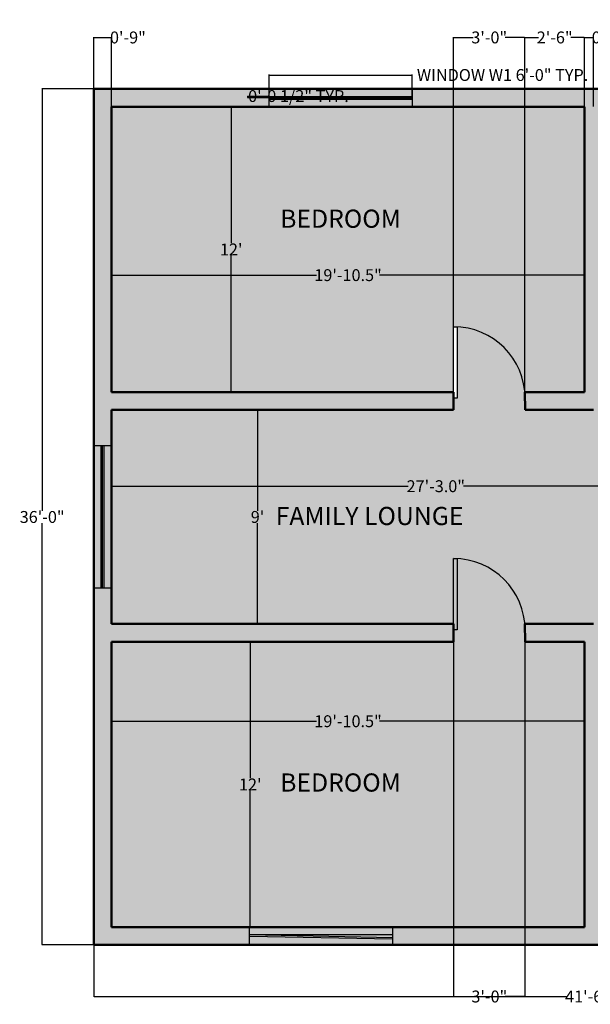
# Model space of a CAD drawing. Units: inches. Extents: x 1379 to 6665, y -118 to 1026.
# Tile 9 of 29: x 2244 to 2532, y 150 to 647. Entities that reach past the tile are written whole.
import ezdxf

# ---------------------------------------------------------------- set-up
doc = ezdxf.new("R2010")
doc.units = ezdxf.units.IN
doc.header["$MEASUREMENT"] = 0
for name, color, linetype, lineweight in [('A-ANNO-DIMS', 2, 'Continuous', 18), ('A-AREA-IDEN', 7, 'Continuous', 25), ('A-DOOR', 1, 'Continuous', 25), ('A-FLOR-PATT', 252, 'Continuous', 13), ('A-GLAZ', 2, 'Continuous', 25), ('A-WALL', 7, 'Continuous', 50), ('A-WALL-PATT', 8, 'Continuous', 13)]:
    doc.layers.add(name, color=color, linetype=linetype, lineweight=lineweight)
doc.styles.get("Standard").update_dxf_attribs({"font": 'arial.ttf'})
doc.dimstyles.get("Standard").update_dxf_attribs({"dimtxt": 6, "dimasz": 0.18, "dimexe": 0.18, "dimexo": 0.0625, "dimgap": 0.09, "dimtad": 0, "dimtih": 1, "dimtoh": 1, "dimdec": 1, "dimzin": 0, "dimdsep": 46, "dimlunit": 3, "dimtxsty": 'Standard', "dimcen": 0.09, "dimclrt": 250, "dimadec": 0, "dimazin": 0, "dimtfac": 1, "dimtdec": 1, "dimtofl": 0, "dimtmove": 0, "dimatfit": 3, "dimfxl": 1, "dimtolj": 1, "dimtzin": 0, "dimarcsym": 0})

# ---------------------------------------------------------------- blocks, each defined once
blk = doc.blocks.new('*U3')
for p, q in [((0, 0), (0, -6)), ((36, 0), (36, -6))]:
    blk.add_line(p, q)
blk.add_lwpolyline([(0, 0), (0, 36), (1.75, 36), (1.75, 0)], close=True)
blk.add_arc((0, 0), 36, 0, 90)
blk = doc.blocks.new('*D26')
at = {"layer": 'A-ANNO-DIMS', "color": 0, "lineweight": -2, "transparency": 16777216}
for p, q in [((2349.32, 602.93), (2350.88, 602.93)), ((2350.7, 602.75), (2350.7, 534.04)), ((2350.7, 459.11), (2350.7, 527.83)), ((2349.32, 458.93), (2350.88, 458.93))]:
    blk.add_line(p, q, dxfattribs=at)
at = {"layer": 'A-ANNO-DIMS', "color": 0, "transparency": 16777216}
for points in [[(2350.67, 602.75), (2350.73, 602.75), (2350.7, 602.93)], [(2350.67, 459.11), (2350.73, 459.11), (2350.7, 458.93)]]:
    blk.add_solid(points, dxfattribs=at)
at = {"layer": 'Defpoints', "color": 0, "transparency": 16777216}
for p in [(2349.26, 602.93), (2349.26, 458.93), (2350.7, 458.93)]:
    blk.add_point(p, dxfattribs=at)
at = {"layer": 'A-ANNO-DIMS', "color": 0, "transparency": 16777216, "insert": (2350.7, 530.93), "char_height": 6, "attachment_point": 5}
blk.add_mtext("\\A1;12'", dxfattribs=at)
blk = doc.blocks.new('*D27')
at = {"layer": 'A-ANNO-DIMS', "color": 0, "lineweight": -2, "transparency": 16777216}
for p, q in [((2290.35, 525.65), (2290.35, 517.8)), ((2528.85, 525.65), (2528.85, 517.8)), ((2290.53, 517.98), (2393.66, 517.98)), ((2528.67, 517.98), (2425.54, 517.98))]:
    blk.add_line(p, q, dxfattribs=at)
at = {"layer": 'A-ANNO-DIMS', "color": 0, "transparency": 16777216}
for points in [[(2290.53, 518.01), (2290.53, 517.95), (2290.35, 517.98)], [(2528.67, 518.01), (2528.67, 517.95), (2528.85, 517.98)]]:
    blk.add_solid(points, dxfattribs=at)
at = {"layer": 'Defpoints', "color": 0, "transparency": 16777216}
for p in [(2290.35, 525.72), (2528.85, 525.72), (2528.85, 517.98)]:
    blk.add_point(p, dxfattribs=at)
at = {"layer": 'A-ANNO-DIMS', "color": 0, "transparency": 16777216, "insert": (2409.6, 517.98), "char_height": 6, "attachment_point": 5}
blk.add_mtext('\\A1;19\'-10.5"', dxfattribs=at)
blk = doc.blocks.new('*D28')
at = {"layer": 'A-ANNO-DIMS', "color": 0, "lineweight": -2, "transparency": 16777216}
for p, q in [((2395.82, 449.93), (2363.77, 449.93)), ((2363.95, 449.75), (2363.95, 399.09)), ((2363.95, 342.11), (2363.95, 392.78)), ((2395.82, 341.93), (2363.77, 341.93))]:
    blk.add_line(p, q, dxfattribs=at)
at = {"layer": 'A-ANNO-DIMS', "color": 0, "transparency": 16777216}
for points in [[(2363.92, 449.75), (2363.98, 449.75), (2363.95, 449.93)], [(2363.92, 342.11), (2363.98, 342.11), (2363.95, 341.93)]]:
    blk.add_solid(points, dxfattribs=at)
at = {"layer": 'Defpoints', "color": 0, "transparency": 16777216}
for p in [(2395.88, 449.93), (2363.95, 341.93), (2395.88, 341.93)]:
    blk.add_point(p, dxfattribs=at)
at = {"layer": 'A-ANNO-DIMS', "color": 0, "transparency": 16777216, "insert": (2363.95, 395.93), "char_height": 6, "attachment_point": 5}
blk.add_mtext("\\A1;9'", dxfattribs=at)
blk = doc.blocks.new('*D29')
at = {"layer": 'A-ANNO-DIMS', "color": 0, "lineweight": -2, "transparency": 16777216}
for p, q in [((2290.35, 390.52), (2290.35, 411.63)), ((2290.53, 411.45), (2439.91, 411.45)), ((2617.17, 411.45), (2467.79, 411.45)), ((2617.35, 390.52), (2617.35, 411.63))]:
    blk.add_line(p, q, dxfattribs=at)
at = {"layer": 'A-ANNO-DIMS', "color": 0, "transparency": 16777216}
for points in [[(2290.53, 411.48), (2290.53, 411.42), (2290.35, 411.45)], [(2617.17, 411.48), (2617.17, 411.42), (2617.35, 411.45)]]:
    blk.add_solid(points, dxfattribs=at)
at = {"layer": 'Defpoints', "color": 0, "transparency": 16777216}
for p in [(2617.35, 411.45), (2290.35, 390.45), (2617.35, 390.45)]:
    blk.add_point(p, dxfattribs=at)
at = {"layer": 'A-ANNO-DIMS', "color": 0, "transparency": 16777216, "insert": (2453.85, 411.45), "char_height": 6, "attachment_point": 5}
blk.add_mtext('\\A1;27\'-3.0"', dxfattribs=at)
blk = doc.blocks.new('*D36')
at = {"layer": 'A-ANNO-DIMS', "color": 0, "lineweight": -2, "transparency": 16777216}
for p, q in [((2376.54, 332.93), (2360.12, 332.93)), ((2360.3, 332.75), (2360.3, 264.04)), ((2360.3, 189.11), (2360.3, 257.83)), ((2376.54, 188.93), (2360.12, 188.93))]:
    blk.add_line(p, q, dxfattribs=at)
at = {"layer": 'A-ANNO-DIMS', "color": 0, "transparency": 16777216}
for points in [[(2360.27, 332.75), (2360.33, 332.75), (2360.3, 332.93)], [(2360.27, 189.11), (2360.33, 189.11), (2360.3, 188.93)]]:
    blk.add_solid(points, dxfattribs=at)
at = {"layer": 'Defpoints', "color": 0, "transparency": 16777216}
for p in [(2376.6, 332.93), (2360.3, 188.93), (2376.6, 188.93)]:
    blk.add_point(p, dxfattribs=at)
at = {"layer": 'A-ANNO-DIMS', "color": 0, "transparency": 16777216, "insert": (2360.3, 260.93), "char_height": 6, "attachment_point": 5}
blk.add_mtext("\\A1;12'", dxfattribs=at)
blk = doc.blocks.new('*D37')
at = {"layer": 'A-ANNO-DIMS', "color": 0, "lineweight": -2, "transparency": 16777216}
for p, q in [((2290.35, 271.73), (2290.35, 293.03)), ((2290.53, 292.85), (2393.66, 292.85)), ((2528.67, 292.85), (2425.54, 292.85)), ((2528.85, 273), (2528.85, 293.03))]:
    blk.add_line(p, q, dxfattribs=at)
at = {"layer": 'A-ANNO-DIMS', "color": 0, "transparency": 16777216}
for points in [[(2290.53, 292.88), (2290.53, 292.82), (2290.35, 292.85)], [(2528.67, 292.88), (2528.67, 292.82), (2528.85, 292.85)]]:
    blk.add_solid(points, dxfattribs=at)
at = {"layer": 'Defpoints', "color": 0, "transparency": 16777216}
for p in [(2528.85, 292.85), (2290.35, 271.66), (2528.85, 272.93)]:
    blk.add_point(p, dxfattribs=at)
at = {"layer": 'A-ANNO-DIMS', "color": 0, "transparency": 16777216, "insert": (2409.6, 292.85), "char_height": 6, "attachment_point": 5}
blk.add_mtext('\\A1;19\'-10.5"', dxfattribs=at)
blk = doc.blocks.new('WIN-1800')
for p, q in [((0, 0.73), (72, 0.73)), ((0, 0), (72, 0))]:
    blk.add_line(p, q)
blk = doc.blocks.new('*D111')
at = {"layer": 'A-ANNO-DIMS', "color": 0, "lineweight": -2, "transparency": 16777216}
for p, q in [((2369.85, 608.23), (2369.85, 619.15)), ((2370.03, 618.97), (2441.67, 618.97)), ((2441.85, 608.23), (2441.85, 619.15)), ((2441.85, 618.97), (2442.03, 618.97))]:
    blk.add_line(p, q, dxfattribs=at)
at = {"layer": 'A-ANNO-DIMS', "color": 0, "transparency": 16777216}
for points in [[(2370.03, 619), (2370.03, 618.94), (2369.85, 618.97)], [(2441.67, 619), (2441.67, 618.94), (2441.85, 618.97)]]:
    blk.add_solid(points, dxfattribs=at)
at = {"layer": 'Defpoints', "color": 0, "transparency": 16777216}
for p in [(2441.85, 618.97), (2369.85, 608.17), (2441.85, 608.17)]:
    blk.add_point(p, dxfattribs=at)
at = {"layer": 'A-ANNO-DIMS', "color": 250, "transparency": 16777216, "insert": (2487.53, 618.97), "char_height": 6, "attachment_point": 5}
blk.add_mtext('\\A1;WINDOW W1 6\'-0" TYP.', dxfattribs=at)
blk = doc.blocks.new('*D112')
at = {"layer": 'A-ANNO-DIMS', "color": 0, "lineweight": -2, "transparency": 16777216}
for p, q in [((2369.79, 608.17), (2358.87, 608.17)), ((2369.79, 607.43), (2358.87, 607.43)), ((2359.05, 608.17), (2359.05, 608.35)), ((2359.05, 608.35), (2359.23, 608.35)), ((2359.05, 607.61), (2359.05, 607.99))]:
    blk.add_line(p, q, dxfattribs=at)
at = {"layer": 'A-ANNO-DIMS', "color": 0, "transparency": 16777216}
for points in [[(2359.02, 607.99), (2359.08, 607.99), (2359.05, 608.17)], [(2359.02, 607.61), (2359.08, 607.61), (2359.05, 607.43)]]:
    blk.add_solid(points, dxfattribs=at)
at = {"layer": 'Defpoints', "color": 0, "transparency": 16777216}
for p in [(2359.05, 608.17), (2369.85, 608.17), (2369.85, 607.43)]:
    blk.add_point(p, dxfattribs=at)
at = {"layer": 'A-ANNO-DIMS', "color": 250, "transparency": 16777216, "insert": (2384.6, 608.35), "char_height": 6, "attachment_point": 5}
blk.add_mtext('\\A1;0\'-0 1/2" TYP.', dxfattribs=at)
blk = doc.blocks.new('*D152')
at = {"layer": 'A-ANNO-DIMS', "color": 0, "lineweight": -2, "transparency": 16777216}
for p, q in [((2281.35, 179.87), (2281.35, 153.75)), ((2779.35, 179.87), (2779.35, 153.75)), ((2281.53, 153.93), (2519.83, 153.93)), ((2779.17, 153.93), (2540.87, 153.93))]:
    blk.add_line(p, q, dxfattribs=at)
at = {"layer": 'A-ANNO-DIMS', "color": 0, "transparency": 16777216}
for points in [[(2281.53, 153.96), (2281.53, 153.9), (2281.35, 153.93)], [(2779.17, 153.96), (2779.17, 153.9), (2779.35, 153.93)]]:
    blk.add_solid(points, dxfattribs=at)
at = {"layer": 'Defpoints', "color": 0, "transparency": 16777216}
for p in [(2281.35, 179.93), (2779.35, 179.93), (2779.35, 153.93)]:
    blk.add_point(p, dxfattribs=at)
at = {"layer": 'A-ANNO-DIMS', "color": 250, "transparency": 16777216, "insert": (2530.35, 153.93), "char_height": 6, "attachment_point": 5}
blk.add_mtext('\\A1;41\'-6"', dxfattribs=at)
blk = doc.blocks.new('*D153')
at = {"layer": 'A-ANNO-DIMS', "color": 0, "lineweight": -2, "transparency": 16777216}
for p, q in [((2281.29, 611.93), (2255.17, 611.93)), ((2255.35, 611.75), (2255.35, 399.09)), ((2255.35, 180.11), (2255.35, 392.78)), ((2281.29, 179.93), (2255.17, 179.93))]:
    blk.add_line(p, q, dxfattribs=at)
at = {"layer": 'A-ANNO-DIMS', "color": 0, "transparency": 16777216}
for points in [[(2255.32, 611.75), (2255.38, 611.75), (2255.35, 611.93)], [(2255.32, 180.11), (2255.38, 180.11), (2255.35, 179.93)]]:
    blk.add_solid(points, dxfattribs=at)
at = {"layer": 'Defpoints', "color": 0, "transparency": 16777216}
for p in [(2255.35, 611.93), (2281.35, 611.93), (2281.35, 179.93)]:
    blk.add_point(p, dxfattribs=at)
at = {"layer": 'A-ANNO-DIMS', "color": 250, "transparency": 16777216, "insert": (2255.35, 395.93), "char_height": 6, "attachment_point": 5}
blk.add_mtext('\\A1;36\'-0"', dxfattribs=at)
blk = doc.blocks.new('*D154')
at = {"layer": 'A-ANNO-DIMS', "color": 0, "lineweight": -2, "transparency": 16777216}
for p, q in [((2281.35, 612), (2281.35, 638.11)), ((2281.53, 637.93), (2290.17, 637.93)), ((2290.35, 603), (2290.35, 638.11)), ((2290.35, 637.93), (2290.53, 637.93))]:
    blk.add_line(p, q, dxfattribs=at)
at = {"layer": 'A-ANNO-DIMS', "color": 0, "transparency": 16777216}
for points in [[(2281.53, 637.96), (2281.53, 637.9), (2281.35, 637.93)], [(2290.17, 637.96), (2290.17, 637.9), (2290.35, 637.93)]]:
    blk.add_solid(points, dxfattribs=at)
at = {"layer": 'Defpoints', "color": 0, "transparency": 16777216}
for p in [(2290.35, 637.93), (2281.35, 611.93), (2290.35, 602.93)]:
    blk.add_point(p, dxfattribs=at)
at = {"layer": 'A-ANNO-DIMS', "color": 250, "transparency": 16777216, "insert": (2298.6, 637.93), "char_height": 6, "attachment_point": 5}
blk.add_mtext('\\A1;0\'-9"', dxfattribs=at)
blk = doc.blocks.new('*D155')
at = {"layer": 'A-ANNO-DIMS', "color": 0, "lineweight": -2, "transparency": 16777216}
for p, q in [((2528.85, 603), (2528.85, 638.11)), ((2529.03, 637.93), (2533.17, 637.93)), ((2533.35, 603), (2533.35, 638.11)), ((2533.35, 637.93), (2533.53, 637.93))]:
    blk.add_line(p, q, dxfattribs=at)
at = {"layer": 'A-ANNO-DIMS', "color": 0, "transparency": 16777216}
for points in [[(2529.03, 637.96), (2529.03, 637.9), (2528.85, 637.93)], [(2533.17, 637.96), (2533.17, 637.9), (2533.35, 637.93)]]:
    blk.add_solid(points, dxfattribs=at)
at = {"layer": 'Defpoints', "color": 0, "transparency": 16777216}
for p in [(2533.35, 637.93), (2528.85, 602.93), (2533.35, 602.93)]:
    blk.add_point(p, dxfattribs=at)
at = {"layer": 'A-ANNO-DIMS', "color": 250, "transparency": 16777216, "insert": (2548.59, 637.93), "char_height": 6, "attachment_point": 5}
blk.add_mtext('\\A1;0\'-4 1/2"', dxfattribs=at)
blk = doc.blocks.new('*D159')
at = {"layer": 'A-ANNO-DIMS', "color": 0, "lineweight": -2, "transparency": 16777216}
for p, q in [((2498.73, 459), (2498.73, 638.11)), ((2498.91, 637.93), (2505.67, 637.93)), ((2528.67, 637.93), (2521.9, 637.93)), ((2528.85, 459), (2528.85, 638.11))]:
    blk.add_line(p, q, dxfattribs=at)
at = {"layer": 'A-ANNO-DIMS', "color": 0, "transparency": 16777216}
for points in [[(2498.91, 637.96), (2498.91, 637.9), (2498.73, 637.93)], [(2528.67, 637.96), (2528.67, 637.9), (2528.85, 637.93)]]:
    blk.add_solid(points, dxfattribs=at)
at = {"layer": 'Defpoints', "color": 0, "transparency": 16777216}
for p in [(2528.85, 637.93), (2498.73, 458.93), (2528.85, 458.93)]:
    blk.add_point(p, dxfattribs=at)
at = {"layer": 'A-ANNO-DIMS', "color": 250, "transparency": 16777216, "insert": (2513.79, 637.93), "char_height": 6, "attachment_point": 5}
blk.add_mtext('\\A1;2\'-6"', dxfattribs=at)
blk = doc.blocks.new('*D160')
at = {"layer": 'A-ANNO-DIMS', "color": 0, "lineweight": -2, "transparency": 16777216}
for p, q in [((2462.85, 459), (2462.85, 638.11)), ((2463.03, 637.93), (2472.73, 637.93)), ((2498.55, 637.93), (2488.85, 637.93)), ((2498.73, 459), (2498.73, 638.11))]:
    blk.add_line(p, q, dxfattribs=at)
at = {"layer": 'A-ANNO-DIMS', "color": 0, "transparency": 16777216}
for points in [[(2463.03, 637.96), (2463.03, 637.9), (2462.85, 637.93)], [(2498.55, 637.96), (2498.55, 637.9), (2498.73, 637.93)]]:
    blk.add_solid(points, dxfattribs=at)
at = {"layer": 'Defpoints', "color": 0, "transparency": 16777216}
for p in [(2498.73, 637.93), (2462.85, 458.93), (2498.73, 458.93)]:
    blk.add_point(p, dxfattribs=at)
at = {"layer": 'A-ANNO-DIMS', "color": 250, "transparency": 16777216, "insert": (2480.79, 637.93), "char_height": 6, "attachment_point": 5}
blk.add_mtext('\\A1;3\'-0"', dxfattribs=at)
blk = doc.blocks.new('*D161')
at = {"layer": 'A-ANNO-DIMS', "color": 0, "lineweight": -2, "transparency": 16777216}
for p, q in [((2462.85, 341.87), (2462.85, 153.75)), ((2498.82, 341.87), (2498.82, 153.75)), ((2463.03, 153.93), (2472.77, 153.93)), ((2498.64, 153.93), (2488.9, 153.93))]:
    blk.add_line(p, q, dxfattribs=at)
at = {"layer": 'A-ANNO-DIMS', "color": 0, "transparency": 16777216}
for points in [[(2463.03, 153.96), (2463.03, 153.9), (2462.85, 153.93)], [(2498.64, 153.96), (2498.64, 153.9), (2498.82, 153.93)]]:
    blk.add_solid(points, dxfattribs=at)
at = {"layer": 'Defpoints', "color": 0, "transparency": 16777216}
for p in [(2462.85, 341.93), (2498.82, 341.93), (2498.82, 153.93)]:
    blk.add_point(p, dxfattribs=at)
at = {"layer": 'A-ANNO-DIMS', "color": 250, "transparency": 16777216, "insert": (2480.83, 153.93), "char_height": 6, "attachment_point": 5}
blk.add_mtext('\\A1;3\'-0"', dxfattribs=at)

msp = doc.modelspace()

# ---------------------------------------------------------------- hatches: boundary and pattern name
at = {"layer": 'A-FLOR-PATT', "transparency": 33554590}
h = msp.add_hatch(color=256, dxfattribs=at)
h.dxf.hatch_style = 1
h.paths.add_polyline_path([(2290.35, 490.43), (2290.35, 602.93), (2369.85, 602.93), (2369.85, 611.93), (2281.35, 611.93), (2281.35, 499.43), (2281.35, 431.93), (2290.35, 431.93), (2290.35, 449.93), (2462.85, 449.93), (2462.85, 458.93), (2290.35, 458.93)])
h.paths.add_polyline_path([(2462.85, 341.93), (2290.35, 341.93), (2290.35, 359.93), (2281.35, 359.93), (2281.35, 179.93), (2359.96, 179.93), (2359.96, 188.93), (2290.35, 188.93), (2290.35, 332.93), (2462.85, 332.93)])
h.paths.add_polyline_path([(2557.35, 188.93), (2533.35, 188.93), (2533.35, 272.93), (2581.35, 272.93), (2581.35, 277.43), (2533.35, 277.43), (2533.35, 332.93), (2533.35, 341.93), (2498.82, 341.93), (2498.85, 332.93), (2528.85, 332.93), (2528.85, 188.93), (2431.96, 188.93), (2431.96, 179.93), (2557.35, 179.93)])
h.paths.add_polyline_path([(2666.85, 188.93), (2614.35, 188.93), (2614.35, 277.43), (2605.35, 277.43), (2605.35, 272.93), (2605.35, 188.93), (2581.35, 188.93), (2581.35, 179.93), (2617.35, 179.93), (2666.85, 179.93)])
h.paths.add_polyline_path([(2779.35, 296.93), (2770.35, 296.93), (2770.35, 284.93), (2740.35, 284.93), (2740.35, 280.43), (2770.35, 280.43), (2770.35, 188.93), (2738.85, 188.93), (2738.85, 179.93), (2779.35, 179.93)])
h.paths.add_polyline_path([(2779.35, 611.93), (2728.35, 611.93), (2728.35, 602.93), (2770.35, 602.93), (2770.35, 482.93), (2722.35, 482.93), (2722.35, 478.43), (2770.35, 478.43), (2770.35, 439.43), (2626.35, 439.43), (2617.35, 439.43), (2617.35, 430.43), (2617.35, 425.93), (2770.35, 425.93), (2770.35, 341.93), (2617.35, 341.93), (2569.35, 341.93), (2569.35, 332.93), (2617.35, 332.93), (2681.85, 332.93), (2681.85, 284.93), (2654.35, 284.93), (2654.35, 280.43), (2681.85, 280.43), (2716.35, 280.43), (2716.35, 284.93), (2686.35, 284.93), (2686.35, 332.93), (2770.35, 332.93), (2770.35, 320.93), (2779.35, 320.93)])
h.paths.add_polyline_path([(2698.35, 482.93), (2650.35, 482.93), (2650.35, 478.43), (2650.35, 439.43), (2654.85, 439.43), (2654.85, 478.43), (2698.35, 478.43)], flags=17)
h.paths.add_polyline_path([(2614.35, 602.93), (2656.35, 602.93), (2656.35, 611.93), (2581.35, 611.93), (2581.35, 602.93), (2605.35, 602.93), (2605.35, 478.43), (2614.35, 478.43), (2614.35, 482.93)], flags=17)
h.paths.add_polyline_path([(2557.35, 611.93), (2521.35, 611.93), (2441.85, 611.93), (2441.85, 602.93), (2521.35, 602.93), (2528.85, 602.93), (2528.85, 458.93), (2498.73, 458.93), (2498.85, 449.93), (2533.35, 449.93), (2533.35, 514.43), (2581.35, 514.43), (2581.35, 518.93), (2533.35, 518.93), (2533.35, 602.93), (2557.35, 602.93)])
at = {"layer": 'A-WALL-PATT', "transparency": 33554564}
h = msp.add_hatch(color=256, dxfattribs=at)
h.dxf.hatch_style = 1
h.paths.add_polyline_path([(2441.85, 611.93), (2369.85, 611.93), (2369.85, 608.17), (2441.85, 608.17)])
h.paths.add_polyline_path([(2441.85, 607.43), (2369.85, 607.43), (2369.85, 606.7), (2441.85, 606.7)])
h.paths.add_polyline_path([(2441.85, 608.17), (2369.85, 608.17), (2369.85, 607.43), (2441.85, 607.43)])
h.paths.add_polyline_path([(2441.85, 606.7), (2369.85, 606.7), (2369.85, 602.93), (2441.85, 602.93)])
at = {"layer": 'A-WALL-PATT', "transparency": 33554590}
h = msp.add_hatch(color=256, dxfattribs=at)
h.dxf.hatch_style = 1
h.paths.add_polyline_path([(2528.85, 602.93), (2290.35, 602.93), (2290.35, 490.43), (2290.35, 458.93), (2462.85, 458.93), (2462.85, 491.93), (2464.6, 491.93), (2464.6, 491.89, -0.376042), (2498.73, 458.93), (2528.85, 458.93)])
h.paths.add_polyline_path([(2617.35, 425.93), (2617.35, 430.43), (2617.35, 439.43), (2626.35, 439.43), (2650.35, 439.43), (2650.35, 478.43), (2650.35, 484.43, 0.400041), (2616.1, 520.39), (2616.1, 484.43), (2614.35, 484.43), (2614.35, 478.43), (2605.35, 478.43), (2605.35, 522.68, 0.392996), (2583.1, 546.62), (2583.1, 522.68), (2581.35, 522.68), (2581.35, 516.68), (2581.35, 514.43), (2533.35, 514.43), (2533.35, 449.93), (2498.85, 449.93), (2498.73, 458.93, 0.376042), (2464.6, 491.89), (2464.6, 455.93), (2462.85, 455.93), (2462.85, 449.93), (2290.35, 449.93), (2290.35, 341.93), (2462.85, 341.93), (2462.85, 374.93), (2464.6, 374.93), (2464.6, 374.89, -0.376042), (2498.73, 341.93), (2533.35, 341.93), (2533.35, 332.93), (2533.35, 277.43), (2581.35, 277.43), (2581.35, 281.18), (2581.35, 305.18), (2583.1, 305.18), (2583.1, 305.12, -0.392996), (2605.35, 281.18), (2605.35, 277.43), (2614.35, 277.43), (2614.35, 283.43), (2614.35, 323.43), (2616.1, 323.43), (2616.1, 323.4, -0.390605), (2654.32, 284.93), (2681.85, 284.93), (2681.85, 332.93), (2614.35, 332.93), (2569.35, 332.93), (2569.35, 341.93), (2617.35, 341.93), (2617.35, 383.93)])
h.paths.add_polyline_path([(2605.35, 602.93), (2533.35, 602.93), (2533.35, 518.93), (2581.35, 518.93), (2581.35, 522.68), (2581.35, 546.68), (2583.1, 546.68), (2583.1, 546.62, -0.392996), (2605.35, 522.68)])
h.paths.add_polyline_path([(2770.35, 602.93), (2614.35, 602.93), (2614.35, 520.43), (2616.1, 520.43), (2616.1, 520.39, -0.400041), (2650.35, 484.43), (2650.35, 482.93), (2698.35, 482.93), (2698.35, 484.43), (2698.35, 508.43), (2700.1, 508.43), (2700.1, 508.37, -0.392996), (2722.35, 484.43), (2722.35, 482.93), (2770.35, 482.93)])
h.paths.add_polyline_path([(2528.85, 332.93), (2498.85, 332.93), (2498.82, 341.93), (2498.73, 341.93, 0.376042), (2464.6, 374.89), (2464.6, 374.93), (2462.85, 374.93), (2462.85, 341.93), (2462.85, 332.93), (2290.35, 332.93), (2290.35, 188.93), (2528.85, 188.93)])
h.paths.add_polyline_path([(2605.35, 272.93), (2605.35, 277.43), (2605.35, 281.18, 0.392996), (2583.1, 305.12), (2583.1, 281.18), (2581.35, 281.18), (2581.35, 277.43), (2581.35, 275.18), (2581.35, 272.93), (2533.35, 272.93), (2533.35, 188.93), (2605.35, 188.93)])
h.paths.add_polyline_path([(2770.35, 280.43), (2740.35, 280.43), (2740.35, 286.43, 0.392996), (2718.1, 310.37), (2718.1, 286.43), (2716.35, 286.43), (2716.35, 280.43), (2681.85, 280.43), (2654.35, 280.43), (2654.35, 283.43, 0.401453), (2616.1, 323.4), (2616.1, 283.43), (2614.35, 283.43), (2614.35, 277.43), (2614.35, 188.93), (2617.35, 188.93), (2770.35, 188.93)])
h.paths.add_polyline_path([(2770.35, 332.93), (2686.35, 332.93), (2686.35, 284.93), (2716.35, 284.93), (2716.35, 286.43), (2716.35, 310.43), (2718.1, 310.43), (2718.1, 310.37, -0.392996), (2740.35, 286.43), (2740.35, 284.93), (2770.35, 284.93)])
h.paths.add_polyline_path([(2770.35, 478.43), (2722.35, 478.43), (2722.35, 484.43, 0.392996), (2700.1, 508.37), (2700.1, 484.43), (2698.35, 484.43), (2698.35, 482.93), (2698.35, 478.43), (2654.85, 478.43), (2654.85, 439.43), (2770.35, 439.43)])
h.paths.add_polyline_path([(2372.98, 539.34), (2443.91, 539.34), (2443.91, 553.57), (2372.98, 553.57)], flags=24)
h.paths.add_polyline_path([(2370.72, 389.31), (2479.4, 389.31), (2479.4, 403.55), (2370.72, 403.55)], flags=24)
h.paths.add_polyline_path([(2550.99, 562.74), (2600.58, 562.74), (2600.58, 576.98), (2550.99, 576.98)], flags=24)
h.paths.add_polyline_path([(2663.19, 559.03), (2734.13, 559.03), (2734.13, 573.27), (2663.19, 573.27)], flags=24)
h.paths.add_polyline_path([(2372.98, 254.81), (2443.91, 254.81), (2443.91, 269.04), (2372.98, 269.04)], flags=24)
h.paths.add_polyline_path([(2545.25, 230.45), (2594.84, 230.45), (2594.84, 244.68), (2545.25, 244.68)], flags=24)
h.paths.add_polyline_path([(2664.48, 230.74), (2735.42, 230.74), (2735.42, 244.97), (2664.48, 244.97)], flags=24)
h.paths.add_polyline_path([(2704.72, 315.06), (2754.31, 315.06), (2754.31, 329.29), (2704.72, 329.29)], flags=24)
h.paths.add_polyline_path([(2688.89, 449.86), (2738.48, 449.86), (2738.48, 464.09), (2688.89, 464.09)], flags=24)
at = {"layer": 'A-WALL-PATT', "transparency": 33554564}
h = msp.add_hatch(color=256, dxfattribs=at)
h.dxf.hatch_style = 1
h.paths.add_polyline_path([(2281.35, 431.93), (2281.35, 359.93), (2285.12, 359.93), (2285.12, 431.93)])
h.paths.add_polyline_path([(2285.85, 431.93), (2285.85, 359.93), (2286.58, 359.93), (2286.58, 431.93)])
h.paths.add_polyline_path([(2285.12, 431.93), (2285.12, 359.93), (2285.85, 359.93), (2285.85, 431.93)])
h.paths.add_polyline_path([(2286.58, 431.93), (2286.58, 359.93), (2290.35, 359.93), (2290.35, 431.93)])
h = msp.add_hatch(color=256, dxfattribs=at)
h.dxf.hatch_style = 1
h.paths.add_polyline_path([(2431.96, 188.93), (2359.96, 188.93), (2359.96, 185.17), (2431.96, 185.17)])
h.paths.add_polyline_path([(2431.96, 184.43), (2359.96, 184.43), (2359.96, 183.7), (2431.96, 183.7)])
h.paths.add_polyline_path([(2431.96, 185.17), (2359.96, 185.17), (2359.96, 184.43), (2431.96, 184.43)])
h.paths.add_polyline_path([(2431.96, 183.7), (2359.96, 183.7), (2359.96, 179.93), (2431.96, 179.93)])

# ---------------------------------------------------------------- linework, layer by layer
at = {"layer": 'A-GLAZ'}
for p, q in [((2369.85, 606.7), (2441.85, 606.7)), ((2285.12, 359.93), (2285.12, 431.93)), ((2285.85, 359.93), (2285.85, 431.93)), ((2286.58, 359.93), (2286.58, 431.93)), ((2359.96, 185.17), (2431.96, 185.17))]:
    msp.add_line(p, q, dxfattribs=at)
for points in [[(2369.85, 611.93), (2441.85, 611.93), (2441.85, 602.93), (2369.85, 602.93)], [(2281.35, 359.93), (2281.35, 431.93), (2290.35, 431.93), (2290.35, 359.93)], [(2359.96, 188.93), (2431.96, 188.93), (2431.96, 179.93), (2359.96, 179.93)]]:
    msp.add_lwpolyline(points, close=True, dxfattribs=at)
at = {"layer": 'A-WALL'}
for p, q in [((2281.35, 499.43), (2281.35, 611.93)), ((2281.35, 611.93), (2521.35, 611.93)), ((2779.35, 611.93), (2521.35, 611.93)), ((2290.35, 602.93), (2521.35, 602.93)), ((2290.35, 490.43), (2290.35, 602.93)), ((2528.85, 602.93), (2290.35, 602.93)), ((2528.85, 458.93), (2528.85, 602.93)), ((2281.35, 499.43), (2281.35, 179.93)), ((2290.35, 490.43), (2290.35, 458.93)), ((2462.85, 458.93), (2290.35, 458.93)), ((2462.85, 449.93), (2462.85, 458.93)), ((2528.85, 458.93), (2498.73, 458.93)), ((2498.85, 449.93), (2498.73, 458.93)), ((2462.85, 449.93), (2290.35, 449.93)), ((2290.35, 449.93), (2290.35, 341.93)), ((2533.35, 449.93), (2498.85, 449.93)), ((2462.85, 341.93), (2290.35, 341.93)), ((2462.85, 332.93), (2462.85, 341.93)), ((2533.35, 341.93), (2498.82, 341.93)), ((2498.82, 341.93), (2498.85, 332.93)), ((2462.85, 332.93), (2290.35, 332.93)), ((2290.35, 332.93), (2290.35, 188.93)), ((2528.85, 332.93), (2498.85, 332.93)), ((2528.85, 332.93), (2528.85, 188.93)), ((2528.85, 188.93), (2290.35, 188.93)), ((2617.35, 179.93), (2281.35, 179.93))]:
    msp.add_line(p, q, dxfattribs=at)

# ---------------------------------------------------------------- block references
at = {"layer": 'A-DOOR'}
for p in [(2462.85, 455.93), (2462.85, 338.93)]:
    msp.add_blockref('*U3', p, dxfattribs=at)
at = {"layer": 'A-GLAZ'}
msp.add_blockref('WIN-1800', (2369.85, 607.43), dxfattribs=at)
at = {"layer": 'A-GLAZ', "rotation": 358.834332312017}
msp.add_blockref('WIN-1800', (2359.96, 184.43), dxfattribs=at)

# ---------------------------------------------------------------- texts
at = {"layer": 'A-AREA-IDEN'}
for s, height, p in [('BEDROOM', 9.17, (2375.35, 541.87)), ('FAMILY LOUNGE', 9.1702, (2373.1, 391.84)), ('BEDROOM', 9.17, (2375.35, 257.34))]:
    msp.add_text(s, height=height, dxfattribs=at).set_placement(p)

# ---------------------------------------------------------------- dimensions: what is measured, and where the dimension line sits
at = {"layer": 'A-ANNO-DIMS'}
for base, p1, p2, override, picture, middle in [((2533.35, 637.93), (2528.85, 602.93), (2533.35, 602.93), {"dimdec": 1, "dimlfac": 1, "dimrnd": 0, "dimzin": 1, "dimdsep": 46, "dimlunit": 4, "dimfrac": 2}, '*D155', (2548.59, 637.93)), ((2290.35, 637.93), (2281.35, 611.93), (2290.35, 602.93), {"dimdec": 1, "dimlfac": 1, "dimrnd": 0, "dimzin": 1, "dimdsep": 46, "dimlunit": 4, "dimfrac": 2}, '*D154', (2298.6, 637.93)), ((2498.73, 637.93), (2462.85, 458.93), (2498.73, 458.93), {"dimdec": 1, "dimlfac": 1, "dimrnd": 0, "dimzin": 1, "dimdsep": 46, "dimlunit": 4, "dimfrac": 2}, '*D160', (2480.79, 637.93)), ((2528.85, 637.93), (2498.73, 458.93), (2528.85, 458.93), {"dimdec": 1, "dimlfac": 1, "dimrnd": 0, "dimzin": 1, "dimdsep": 46, "dimlunit": 4, "dimfrac": 2}, '*D159', (2513.79, 637.93)), ((2528.85, 517.98), (2290.35, 525.72), (2528.85, 525.72), {"dimclrd": 0, "dimclre": 0, "dimclrt": 0}, '*D27', (2409.6, 517.98)), ((2617.35, 411.45), (2290.35, 390.45), (2617.35, 390.45), {"dimclrd": 0, "dimclre": 0, "dimclrt": 0}, '*D29', (2453.85, 411.45)), ((2498.82, 153.93), (2462.85, 341.93), (2498.82, 341.93), {"dimdec": 1, "dimlfac": 1, "dimrnd": 0, "dimzin": 1, "dimdsep": 46, "dimlunit": 4, "dimfrac": 2}, '*D161', (2480.83, 153.93)), ((2528.85, 292.85), (2290.35, 271.66), (2528.85, 272.93), {"dimclrd": 0, "dimclre": 0, "dimclrt": 0}, '*D37', (2409.6, 292.85)), ((2779.35, 153.93), (2281.35, 179.93), (2779.35, 179.93), {"dimdec": 1, "dimlfac": 1, "dimrnd": 0, "dimzin": 1, "dimdsep": 46, "dimlunit": 4, "dimfrac": 2}, '*D152', (2530.35, 153.93))]:
    dim = msp.add_linear_dim(base=base, p1=p1, p2=p2, dimstyle='Standard', override=override, dxfattribs=at)
    dim.commit()
    dim.dimension.update_dxf_attribs({"geometry": picture, "text_midpoint": middle})
dim = msp.add_linear_dim(base=(2441.85, 618.97), p1=(2369.85, 608.17), p2=(2441.85, 608.17), text='WINDOW W1 <> TYP.', dimstyle='Standard', override={"dimdec": 1, "dimrnd": 0, "dimzin": 1, "dimlunit": 4, "dimfrac": 2}, dxfattribs=at)
dim.commit()
dim.dimension.update_dxf_attribs({"geometry": '*D111', "text_midpoint": (2487.53, 618.97)})
dim = msp.add_linear_dim(base=(2359.05, 608.17), p1=(2369.85, 607.43), p2=(2369.85, 608.17), angle=90, text='<> TYP.', dimstyle='Standard', override={"dimdec": 1, "dimrnd": 0, "dimzin": 1, "dimlunit": 4, "dimfrac": 2}, dxfattribs=at)
dim.commit()
dim.dimension.update_dxf_attribs({"geometry": '*D112', "text_midpoint": (2384.6, 608.35)})
for base, p1, p2, override, picture, middle in [((2255.35, 611.93), (2281.35, 179.93), (2281.35, 611.93), {"dimdec": 1, "dimlfac": 1, "dimrnd": 0, "dimzin": 1, "dimdsep": 46, "dimlunit": 4, "dimfrac": 2}, '*D153', (2255.35, 395.93)), ((2350.7, 458.93), (2349.26, 602.93), (2349.26, 458.93), {"dimclrd": 0, "dimclre": 0, "dimclrt": 0}, '*D26', (2350.7, 530.93)), ((2363.95, 341.93), (2395.88, 449.93), (2395.88, 341.93), {"dimclrd": 0, "dimclre": 0, "dimclrt": 0}, '*D28', (2363.95, 395.93)), ((2360.3, 188.93), (2376.6, 332.93), (2376.6, 188.93), {"dimclrd": 0, "dimclre": 0, "dimclrt": 0}, '*D36', (2360.3, 260.93))]:
    dim = msp.add_linear_dim(base=base, p1=p1, p2=p2, angle=90, dimstyle='Standard', override=override, dxfattribs=at)
    dim.commit()
    dim.dimension.update_dxf_attribs({"geometry": picture, "text_midpoint": middle})

doc.saveas('drawing.dxf')
